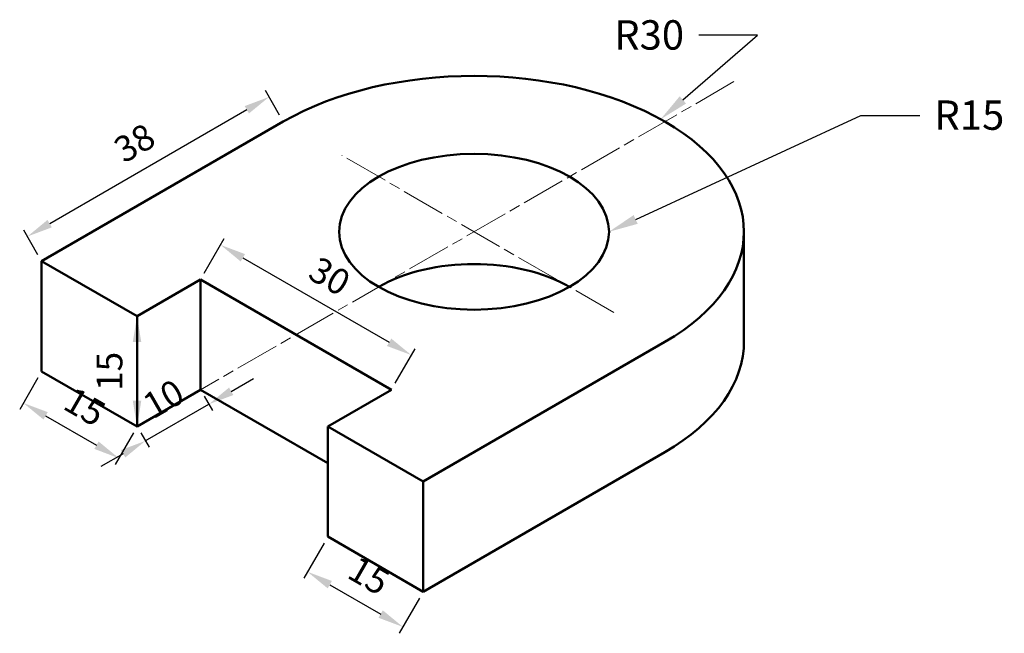
# Model space of a CAD drawing. Units: millimetres. Extents: x 2423 to 2558, y 1182 to 1266.
import ezdxf
from ezdxf import colors
from ezdxf.entities.mleader import LeaderData, LeaderLine
from ezdxf.math import Vec2, Vec3

# ---------------------------------------------------------------- set-up
doc = ezdxf.new("R2010")
doc.units = ezdxf.units.MM
doc.linetypes.add('AM_ISO08W050x2', pattern=[9, 6, -0.75, 1.5, -0.75])
for name, color, linetype, lineweight in [('M-CNTR', 1, 'AM_ISO08W050x2', 18), ('M-DIMS', 3, 'Continuous', 25), ('M-OUTL', 7, 'Continuous', 50)]:
    doc.layers.add(name, color=color, linetype=linetype, lineweight=lineweight)
doc.styles.get("Standard").update_dxf_attribs({"font": 'arial.ttf'})
doc.dimstyles.new('AM_ISO$0', dxfattribs={"dimtxt": 3.5, "dimasz": 3.5, "dimexe": 1, "dimexo": 1, "dimgap": 1.5, "dimtad": 1, "dimdsep": 46, "dimtxsty": 'Standard', "dimcen": 0, "dimclrd": 256, "dimclre": 256, "dimclrt": 2, "dimadec": 0, "dimazin": 2, "dimtp": 0.1, "dimtm": 0.1, "dimtfac": 0.71, "dimtdec": 3, "dimtmove": 0, "dimatfit": 3, "dimfxl": 1, "dimlwd": -1, "dimlwe": -1, "dimarcsym": 1})

# ---------------------------------------------------------------- blocks, each defined once
blk = doc.blocks.new('*D3')
at = {"layer": 'Defpoints', "color": 0, "transparency": 16777216}
for p in [(2448.08, 1230.34), (2476.78, 1220.05), (2474.06, 1215.34)]:
    blk.add_point(p, dxfattribs=at)
at = {"layer": 'M-DIMS', "color": 0, "linetype": 'ByBlock', "transparency": 16777216}
for p, q in [((2448.58, 1231.21), (2451.3, 1235.92)), ((2453.83, 1233.3), (2473.75, 1221.8)), ((2474.56, 1216.21), (2477.28, 1220.92))]:
    blk.add_line(p, q, dxfattribs=at)
at = {"layer": 'M-DIMS', "color": 0, "transparency": 16777216}
for points in [[(2454.12, 1233.8), (2453.54, 1232.79), (2450.8, 1235.05)], [(2474.04, 1222.3), (2473.46, 1221.29), (2476.78, 1220.05)]]:
    blk.add_solid(points, dxfattribs=at)
at = {"layer": 'M-DIMS', "color": 0, "transparency": 16777216, "insert": (2465.43, 1230.4), "char_height": 3.5, "attachment_point": 5, "rotation": 330}
blk.add_mtext('30', dxfattribs=at)
blk = doc.blocks.new('*D4')
at = {"layer": 'Defpoints', "color": 0, "transparency": 16777216}
for p in [(2426.43, 1217.84), (2439.42, 1210.34), (2436.93, 1206.03)]:
    blk.add_point(p, dxfattribs=at)
at = {"layer": 'M-DIMS', "color": 0, "linetype": 'ByBlock', "transparency": 16777216}
for p, q in [((2425.93, 1216.97), (2423.44, 1212.67)), ((2426.97, 1211.78), (2433.9, 1207.78)), ((2438.92, 1209.47), (2436.43, 1205.17))]:
    blk.add_line(p, q, dxfattribs=at)
at = {"layer": 'M-DIMS', "color": 0, "transparency": 16777216}
for points in [[(2427.26, 1212.29), (2426.68, 1211.28), (2423.94, 1213.53)], [(2434.19, 1208.29), (2433.61, 1207.28), (2436.93, 1206.03)]]:
    blk.add_solid(points, dxfattribs=at)
at = {"layer": 'M-DIMS', "color": 0, "transparency": 16777216, "insert": (2432.08, 1212.63), "char_height": 3.5, "attachment_point": 5, "rotation": 330}
blk.add_mtext('15', dxfattribs=at)
blk = doc.blocks.new('*D5')
at = {"layer": 'Defpoints', "color": 0, "transparency": 16777216}
for p in [(2439.42, 1225.34), (2439.42, 1210.34), (2439.42, 1210.34)]:
    blk.add_point(p, dxfattribs=at)
at = {"layer": 'M-DIMS', "color": 0, "linetype": 'ByBlock', "transparency": 16777216}
blk.add_line((2439.42, 1221.84), (2439.42, 1213.84), dxfattribs=at)
at = {"layer": 'M-DIMS', "color": 0, "transparency": 16777216}
for points in [[(2438.84, 1221.84), (2440, 1221.84), (2439.42, 1225.34)], [(2438.84, 1213.84), (2440, 1213.84), (2439.42, 1210.34)]]:
    blk.add_solid(points, dxfattribs=at)
at = {"layer": 'M-DIMS', "color": 0, "transparency": 16777216, "insert": (2436.13, 1217.84), "char_height": 3.5, "attachment_point": 5, "rotation": 90}
blk.add_mtext('15', dxfattribs=at)
blk = doc.blocks.new('*D6')
at = {"layer": 'Defpoints', "color": 0, "transparency": 16777216}
for p in [(2448.08, 1215.34), (2449.21, 1213.37), (2439.42, 1210.34)]:
    blk.add_point(p, dxfattribs=at)
at = {"layer": 'M-DIMS', "color": 0, "linetype": 'ByBlock', "transparency": 16777216}
for p, q in [((2452.25, 1215.12), (2455.28, 1216.87)), ((2448.58, 1214.47), (2449.71, 1212.51)), ((2440.55, 1208.37), (2449.21, 1213.37)), ((2439.92, 1209.47), (2441.05, 1207.51)), ((2437.52, 1206.62), (2434.49, 1204.87))]:
    blk.add_line(p, q, dxfattribs=at)
at = {"layer": 'M-DIMS', "color": 0, "transparency": 16777216}
for points in [[(2451.95, 1215.63), (2452.54, 1214.62), (2449.21, 1213.37)], [(2437.23, 1207.13), (2437.82, 1206.12), (2440.55, 1208.37)]]:
    blk.add_solid(points, dxfattribs=at)
at = {"layer": 'M-DIMS', "color": 0, "transparency": 16777216, "insert": (2443.24, 1213.72), "char_height": 3.5, "attachment_point": 5, "rotation": 30}
blk.add_mtext('10', dxfattribs=at)
blk = doc.blocks.new('*D7')
at = {"layer": 'Defpoints', "color": 0, "transparency": 16777216}
for p in [(2465.4, 1195.34), (2478.39, 1187.84), (2475.63, 1183.05)]:
    blk.add_point(p, dxfattribs=at)
at = {"layer": 'M-DIMS', "color": 0, "linetype": 'ByBlock', "transparency": 16777216}
for p, q in [((2464.9, 1194.47), (2462.14, 1189.69)), ((2465.67, 1188.8), (2472.6, 1184.8)), ((2477.89, 1186.97), (2475.13, 1182.19))]:
    blk.add_line(p, q, dxfattribs=at)
at = {"layer": 'M-DIMS', "color": 0, "transparency": 16777216}
for points in [[(2465.96, 1189.31), (2465.38, 1188.3), (2462.64, 1190.55)], [(2472.89, 1185.31), (2472.3, 1184.3), (2475.63, 1183.05)]]:
    blk.add_solid(points, dxfattribs=at)
at = {"layer": 'M-DIMS', "color": 0, "transparency": 16777216, "insert": (2470.77, 1189.65), "char_height": 3.5, "attachment_point": 5, "rotation": 330}
blk.add_mtext('15', dxfattribs=at)
blk = doc.blocks.new('*D8')
at = {"layer": 'Defpoints', "color": 0, "transparency": 16777216}
for p in [(2459.34, 1251.84), (2424.49, 1236.19), (2426.43, 1232.84)]:
    blk.add_point(p, dxfattribs=at)
at = {"layer": 'M-DIMS', "color": 0, "linetype": 'ByBlock', "transparency": 16777216}
for p, q in [((2458.84, 1252.71), (2456.9, 1256.06)), ((2454.37, 1253.44), (2427.53, 1237.94)), ((2425.93, 1233.71), (2423.99, 1237.06))]:
    blk.add_line(p, q, dxfattribs=at)
at = {"layer": 'M-DIMS', "color": 0, "transparency": 16777216}
for points in [[(2454.08, 1253.95), (2454.66, 1252.94), (2457.4, 1255.19)], [(2427.23, 1238.45), (2427.82, 1237.44), (2424.49, 1236.19)]]:
    blk.add_solid(points, dxfattribs=at)
at = {"layer": 'M-DIMS', "color": 0, "transparency": 16777216, "insert": (2439.3, 1248.54), "char_height": 3.5, "attachment_point": 5, "rotation": 30}
blk.add_mtext('38', dxfattribs=at)

msp = doc.modelspace()

# ---------------------------------------------------------------- linework, layer by layer
at = {"layer": 'M-CNTR'}
for p, q in [((2520.708, 1257.272), (2448.08, 1215.339)), ((2504.368, 1225.841), (2467.33, 1247.225))]:
    msp.add_line(p, q, dxfattribs=at)
at = {"layer": 'M-OUTL'}
for p, q in [((2426.429, 1232.839), (2459.338, 1251.839)), ((2522.06, 1221.673), (2522.06, 1237.005)), ((2439.419, 1225.339), (2426.429, 1232.839)), ((2426.429, 1232.839), (2426.429, 1217.839)), ((2448.08, 1230.339), (2439.419, 1225.339)), ((2474.06, 1215.339), (2448.08, 1230.339)), ((2448.08, 1215.339), (2448.08, 1230.339)), ((2439.419, 1210.339), (2439.419, 1225.339)), ((2478.39, 1202.839), (2511.299, 1221.839)), ((2426.429, 1217.839), (2439.419, 1210.339)), ((2439.419, 1210.339), (2448.08, 1215.339)), ((2448.08, 1215.339), (2465.4, 1205.339)), ((2465.4, 1210.339), (2474.06, 1215.339)), ((2478.39, 1202.839), (2465.4, 1210.339)), ((2465.4, 1210.339), (2465.4, 1195.339)), ((2478.39, 1187.839), (2511.299, 1206.839)), ((2478.39, 1187.839), (2478.39, 1202.839)), ((2465.4, 1195.339), (2478.39, 1187.839))]:
    msp.add_line(p, q, dxfattribs=at)
for centre, major_axis, start_param, end_param in [((2485.319, 1236.839), (-36.742, 0), 2.3561945, 5.4977871), ((2485.319, 1221.839), (18.371, 0), 0.7853982, 2.3561945), ((2485.319, 1221.839), (-36.742, 0), 8.6393798, 9.432609)]:
    msp.add_ellipse(centre, major_axis=major_axis, ratio=0.5773503, start_param=start_param, end_param=end_param, dxfattribs=at)
msp.add_ellipse((2485.319, 1236.839), major_axis=(-18.371, 0), ratio=0.5773503, dxfattribs=at)

# ---------------------------------------------------------------- dimensions: what is measured, and where the dimension line sits
at = {"layer": 'M-DIMS'}
for p1, p2, distance, override, picture, middle in [((2459.338, 1251.839), (2426.429, 1232.839), -3.87, {"dimclrd": 0, "dimclre": 0, "dimclrt": 0}, '*D8', (2439.304, 1248.538)), ((2448.08, 1230.339), (2474.06, 1215.339), 5.438, {"dimpost": '', "dimclrd": 0, "dimclre": 0, "dimclrt": 0}, '*D3', (2465.433, 1230.397)), ((2439.419, 1225.339), (2439.419, 1210.339), 0, {"dimclrd": 0, "dimclre": 0, "dimclrt": 0}, '*D5', (2436.132, 1217.839)), ((2426.429, 1217.839), (2439.419, 1210.339), -4.974, {"dimclrd": 0, "dimclre": 0, "dimclrt": 0}, '*D4', (2432.081, 1212.628)), ((2439.419, 1210.339), (2448.08, 1215.339), -2.27, {"dimclrd": 0, "dimclre": 0, "dimclrt": 0}, '*D6', (2443.241, 1213.72)), ((2465.4, 1195.339), (2478.39, 1187.839), -5.528, {"dimpost": '', "dimclrd": 0, "dimclre": 0, "dimclrt": 0}, '*D7', (2470.775, 1189.649))]:
    dim = msp.add_aligned_dim(p1=p1, p2=p2, distance=distance, dimstyle='AM_ISO$0', override=override, dxfattribs=at)
    dim.commit()
    dim.dimension.update_dxf_attribs({"geometry": picture, "text_midpoint": middle})

# ---------------------------------------------------------------- leaders
ml = msp.add_multileader_mtext('Standard', dxfattribs=at)
ml.set_content('{\\C2;R30}', color=256)
ml.set_leader_properties()
ml.build(insert=Vec2(0, 0))
ctx = ml.context
ctx.base_point, ctx.plane_origin = Vec3(2502.368, 1263.597), Vec3(2510.728, 1252.162)
ctx.text_align_type = 2
notes = []
notes.append((ctx, [(0, (1, 1, 0), (2523.912, 1263.597), (-1, 0), 8, [(0, [(2510.728, 1252.162)], 0, [])])]))
ctx.mtext.insert, ctx.mtext.alignment, ctx.mtext.flow_direction = Vec3(2513.912, 1265.632), 3, 5
ml = msp.add_multileader_mtext('Standard', dxfattribs=at)
ml.set_content('{\\C2;R15}', color=256)
ml.set_leader_properties()
ml.build(insert=Vec2(0, 0))
ctx = ml.context
ctx.base_point, ctx.plane_origin = Vec3(2545.996, 1252.68), Vec3(2503.69, 1236.839)
notes.append((ctx, [(0, (1, 1, 0), (2537.996, 1252.68), (1, 0), 8, [(0, [(2503.69, 1236.839)], 0, [])])]))
ctx.mtext.insert, ctx.mtext.flow_direction = Vec3(2547.996, 1254.714), 5
for ctx, leaders in notes:
    for number, flags, end, landing, length, lines in leaders:
        leader = LeaderData()
        leader.index, (leader.has_last_leader_line, leader.has_dogleg_vector, leader.attachment_direction) = number, flags
        leader.last_leader_point, leader.dogleg_vector, leader.dogleg_length = Vec3(end), Vec3(landing), length
        for number, points, colour, breaks in lines:
            line = LeaderLine()
            line.index, line.vertices, line.color, line.breaks = number, Vec3.list(points), colors.encode_raw_color(colour), breaks
            leader.lines.append(line)
        ctx.leaders.append(leader)

doc.saveas('drawing.dxf')
